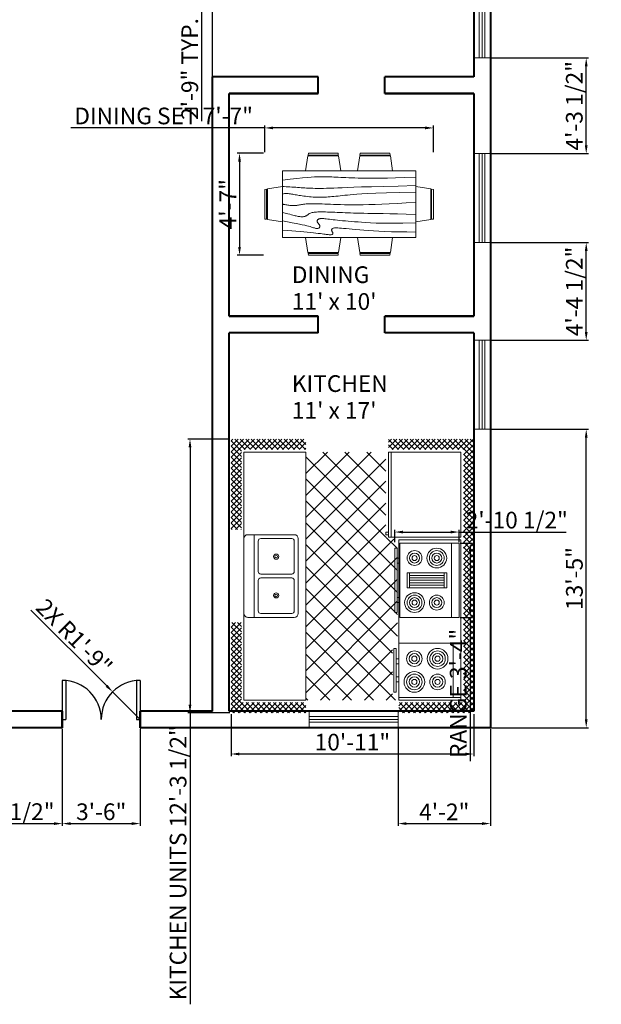
# Model space of a CAD drawing. Units: inches. Extents: x 2383 to 6214, y 970 to 3250.
# Tile 2 of 4: x 2680 to 2994, y 970 to 1500. Entities that reach past the tile are written whole.
import ezdxf

# ---------------------------------------------------------------- set-up
doc = ezdxf.new("R2010")
doc.units = ezdxf.units.IN
for name, color, linetype, lineweight in [('A-ANNO-DIMS', 2, 'Continuous', 18), ('A-AREA-IDEN', 7, 'Continuous', 18), ('A-DOOR', 4, 'Continuous', 25), ('A-EQPM', 8, 'Continuous', 18), ('A-FLOR-FIXT', 8, 'Continuous', 18), ('A-FURN', 8, 'Continuous', 18), ('A-GLAZ', 4, 'Continuous', 18), ('A-WALL', 7, 'Continuous', 40)]:
    doc.layers.add(name, color=color, linetype=linetype, lineweight=lineweight)
doc.styles.get("Standard").update_dxf_attribs({"font": 'arial.ttf'})
doc.dimstyles.new('ISO-25', dxfattribs={"dimtxt": 9, "dimasz": 4.5, "dimexe": 1.25, "dimexo": 0.625, "dimtad": 1, "dimdec": 0, "dimlunit": 3, "dimtxsty": 'Standard', "dimcen": 2.5, "dimadec": 0, "dimazin": 0, "dimtfac": 1, "dimtdec": 0, "dimtmove": 0, "dimatfit": 3, "dimfxl": 1, "dimarcsym": 0})

# ---------------------------------------------------------------- blocks, each defined once
blk = doc.blocks.new('Dining Set - 36 x 72 in.')
for p, q in [((-22, 27.5), (-22.1562, 26.50042)), ((-22, 27.5), (-6, 27.5)), ((-5.8437, 26.49966), (-6, 27.5)), ((6, 27.5), (5.8438, 26.50042)), ((6, 27.5), (22, 27.5)), ((22.1563, 26.49966), (22, 27.5)), ((-22.2343, 26.00059), (-23.4847, 17.99762)), ((-22.2304, 26), (-5.7608, 26)), ((-5.8416, 26.5), (-22.1534, 26.5)), ((-4.5152, 17.99762), (-5.7655, 25.99926)), ((5.7657, 26.00059), (4.5153, 17.99762)), ((5.7696, 26), (22.2392, 26)), ((22.1584, 26.5), (5.8466, 26.5)), ((23.4848, 17.99762), (22.2345, 25.99926)), ((36, 18), (-36, 18)), ((-36, 18), (-36, -18)), ((36, -18), (36, 18)), ((-45.5, 8), (-44.5004, 8.15617)), ((-45.5, 8), (-45.5, -8)), ((-44.5, -8.15843), (-44.5, 8.15338)), ((-44.0006, 8.23428), (-35.9976, 9.48474)), ((-44, 8.23041), (-44, -8.23915)), ((44.0006, 8.23428), (35.9976, 9.48474)), ((44, 8.23041), (44, -8.23915)), ((44.5, -8.15843), (44.5, 8.15338)), ((45.5, 8), (44.5005, 8.15617)), ((45.5, 8), (45.5, -8)), ((-44.4997, -8.15631), (-45.5, -8)), ((-35.9976, -9.48476), (-43.9993, -8.2345)), ((35.9976, -9.48476), (43.9993, -8.2345)), ((44.4997, -8.15631), (45.5, -8)), ((-36, -18), (36, -18)), ((-22.2343, -26.0006), (-23.4847, -17.99762)), ((-4.5152, -17.99762), (-5.7655, -25.99928)), ((5.7657, -26.0006), (4.5153, -17.99762)), ((23.4848, -17.99762), (22.2345, -25.99928)), ((-22.2304, -26), (-5.7608, -26)), ((-22, -27.5), (-22.1562, -26.50044)), ((-5.8416, -26.5), (-22.1534, -26.5)), ((-5.8437, -26.49967), (-6, -27.5)), ((5.7696, -26), (22.2392, -26)), ((6, -27.5), (5.8438, -26.50044)), ((22.1584, -26.5), (5.8466, -26.5)), ((22.1563, -26.49967), (22, -27.5)), ((-22, -27.5), (-6, -27.5)), ((6, -27.5), (22, -27.5))]:
    blk.add_line(p, q)
for points in [[(-36, 15), (-31.1772, 14.97754), (-26.8079, 14.91406), (-22.8538, 14.81543), (-19.276, 14.6875), (-16.0362, 14.53613), (-13.0957, 14.36718), (-10.4159, 14.18652), (-7.9583, 14), (-5.6904, 13.81315), (-3.6035, 13.63021), (-1.6954, 13.45508), (0.0365, 13.29166), (1.5945, 13.14388), (2.9811, 13.01562), (4.1988, 12.9108), (5.25, 12.83333), (6.1393, 12.78613), (6.8802, 12.76823), (7.4883, 12.77767), (7.9792, 12.8125), (8.3685, 12.87077), (8.6719, 12.95052), (8.9049, 13.0498), (9.0833, 13.16666), (9.2205, 13.29899), (9.3216, 13.44401), (9.3895, 13.59879), (9.4271, 13.76041), (9.4373, 13.92594), (9.4232, 14.09245), (9.3875, 14.257), (9.3333, 14.41666), (9.2638, 14.56917), (9.1836, 14.71484), (9.0975, 14.85465), (9.0104, 14.98958), (8.9272, 15.1206), (8.8529, 15.2487), (8.7922, 15.37483), (8.75, 15.5), (8.7305, 15.62467), (8.7344, 15.74739), (8.7617, 15.86621), (8.8125, 15.97916), (8.8867, 16.08431), (8.9844, 16.17968), (9.1055, 16.26334), (9.25, 16.33333), (9.4189, 16.38802), (9.6172, 16.42708), (9.8506, 16.45052), (10.125, 16.45833), (10.4463, 16.45052), (10.8203, 16.42708), (11.2529, 16.38802), (11.75, 16.33333), (12.3184, 16.26318), (12.9694, 16.17838), (13.7151, 16.07991), (14.5677, 15.96875), (15.5395, 15.84586), (16.6426, 15.71224), (17.8893, 15.56884), (19.2917, 15.41666), (20.859, 15.25667), (22.5879, 15.08984), (24.4721, 14.91715), (26.5052, 14.73958), (28.6809, 14.5581), (30.9929, 14.3737), (33.4347, 14.18733), (36, 14)], [(-36, 10), (-28.9766, 10.14274), (-23.1725, 10.20442), (-18.4241, 10.19775), (-14.5677, 10.13541), (-11.4399, 10.03011), (-8.877, 9.89453), (-6.7154, 9.74137), (-4.7917, 9.58333), (-2.9698, 9.43082), (-1.2246, 9.28515), (0.4415, 9.14534), (2.026, 9.01041), (3.5266, 8.87939), (4.9408, 8.7513), (6.266, 8.62516), (7.5, 8.5), (8.6411, 8.37549), (9.6914, 8.2539), (10.6538, 8.13818), (11.5312, 8.03125), (12.3267, 7.93603), (13.043, 7.85547), (13.6831, 7.79248), (14.25, 7.75), (14.7471, 7.7303), (15.1797, 7.73307), (15.5537, 7.75732), (15.875, 7.80208), (16.1494, 7.86637), (16.3828, 7.94922), (16.5811, 8.04964), (16.75, 8.16666), (16.8944, 8.29915), (17.0143, 8.44531), (17.1089, 8.60319), (17.1771, 8.77083), (17.218, 8.94629), (17.2305, 9.1276), (17.2137, 9.31282), (17.1667, 9.5), (17.0895, 9.6875), (16.987, 9.875), (16.8649, 10.0625), (16.7292, 10.25), (16.5856, 10.4375), (16.4401, 10.625), (16.2985, 10.8125), (16.1667, 11), (16.05, 11.18733), (15.9518, 11.3737), (15.8752, 11.5581), (15.8229, 11.73958), (15.798, 11.91715), (15.8034, 12.08984), (15.842, 12.25667), (15.9167, 12.41666), (16.0295, 12.56836), (16.1784, 12.70833), (16.3605, 12.83268), (16.5729, 12.9375), (16.8127, 13.01888), (17.0768, 13.07291), (17.3625, 13.0957), (17.6667, 13.08333), (17.9894, 13.03312), (18.3418, 12.94726), (18.7382, 12.82918), (19.1927, 12.68229), (19.7195, 12.51001), (20.3327, 12.31575), (21.0465, 12.10294), (21.875, 11.875), (22.8357, 11.63354), (23.959, 11.37304), (25.2786, 11.08618), (26.8282, 10.76562), (28.6414, 10.40405), (30.752, 9.99414), (33.1936, 9.52856), (36, 9)], [(-36, 5.5), (-30.7157, 5.3348), (-26.069, 5.20963), (-21.9946, 5.11767), (-18.4271, 5.05208), (-15.3009, 5.00602), (-12.5508, 4.97265), (-10.1112, 4.94515), (-7.9167, 4.91666), (-5.909, 4.88167), (-4.0586, 4.83984), (-2.3429, 4.79215), (-0.7396, 4.73958), (0.7739, 4.6831), (2.22, 4.6237), (3.6213, 4.56233), (5, 4.5), (6.373, 4.43782), (7.7344, 4.3776), (9.0723, 4.32129), (10.375, 4.27083), (11.6309, 4.22819), (12.8281, 4.19531), (13.9551, 4.17415), (15, 4.16666), (15.954, 4.17448), (16.819, 4.19791), (17.6001, 4.23698), (18.3021, 4.29166), (18.9299, 4.36198), (19.4883, 4.44791), (19.9823, 4.54948), (20.4167, 4.66666), (20.7969, 4.79899), (21.1302, 4.94401), (21.4245, 5.09879), (21.6875, 5.26041), (21.9271, 5.42594), (22.1511, 5.59245), (22.3672, 5.757), (22.5834, 5.91666), (22.8065, 6.06868), (23.0404, 6.21093), (23.2879, 6.34147), (23.5521, 6.45833), (23.8358, 6.55957), (24.142, 6.64323), (24.4735, 6.70735), (24.8334, 6.75), (25.2235, 6.76969), (25.642, 6.76692), (26.0858, 6.74267), (26.5521, 6.69791), (27.0379, 6.63362), (27.5404, 6.55078), (28.0565, 6.45036), (28.5834, 6.33333), (29.1242, 6.19987), (29.7071, 6.04687), (30.3661, 5.87044), (31.1354, 5.66666), (32.0493, 5.43164), (33.142, 5.16146), (34.4475, 4.85221), (36, 4.5)], [(-36, -1), (-30.7915, -0.6591), (-26.0195, -0.38216), (-21.6519, -0.16284), (-17.6563, 0.00521), (-14.0005, 0.12833), (-10.6523, 0.21289), (-7.5796, 0.26522), (-4.75, 0.29166), (-2.134, 0.29793), (0.2878, 0.28711), (2.5317, 0.26163), (4.6146, 0.22396), (6.5529, 0.17651), (8.3633, 0.12174), (10.0623, 0.06209), (11.6667, 0), (13.1899, -0.06201), (14.6341, -0.1211), (15.9982, -0.17432), (17.2813, -0.21875), (18.4823, -0.25147), (19.6003, -0.26953), (20.6343, -0.27002), (21.5834, -0.25), (22.4481, -0.20768), (23.2357, -0.14584), (23.9549, -0.06836), (24.6146, 0.02083), (25.2235, 0.11784), (25.7904, 0.21875), (26.3241, 0.31966), (26.8334, 0.41666), (27.3265, 0.50618), (27.8099, 0.58593), (28.2894, 0.65397), (28.7709, 0.70833), (29.2601, 0.74707), (29.763, 0.76823), (30.2855, 0.76985), (30.8334, 0.75), (31.4088, 0.70784), (31.9994, 0.64713), (32.589, 0.57275), (33.1615, 0.48958), (33.7008, 0.4025), (34.1908, 0.3164), (34.6153, 0.23616), (34.9584, 0.16666), (35.2099, 0.11165), (35.3848, 0.07031), (35.504, 0.04069), (35.5886, 0.02083), (35.6594, 0.00879), (35.7377, 0.0026), (35.8442, 0.00032), (36, 0)], [(-36, -6.5), (-27.1843, -6.31267), (-20.084, -6.1263), (-14.469, -5.9419), (-10.1094, -5.76042), (-6.7752, -5.58285), (-4.2363, -5.41016), (-2.2629, -5.24333), (-0.625, -5.08334), (0.8708, -4.93099), (2.2715, -4.78646), (3.5872, -4.64974), (4.8281, -4.52084), (6.0046, -4.39974), (7.127, -4.28646), (8.2053, -4.18099), (9.25, -4.08334), (10.2705, -3.99382), (11.2734, -3.91407), (12.2647, -3.84603), (13.25, -3.79167), (14.2354, -3.75293), (15.2266, -3.73177), (16.2295, -3.73015), (17.25, -3.75), (18.2912, -3.79248), (19.3451, -3.85547), (20.4009, -3.93604), (21.4479, -4.03125), (22.4754, -4.13819), (23.4727, -4.25391), (24.4289, -4.37549), (25.3334, -4.5), (26.1785, -4.62492), (26.9694, -4.74935), (27.7145, -4.87281), (28.4219, -4.99479), (29.1, -5.11483), (29.7572, -5.23242), (30.4016, -5.34709), (31.0417, -5.45834), (31.6837, -5.56437), (32.3262, -5.65821), (32.9658, -5.73153), (33.599, -5.77604), (34.2224, -5.78345), (34.8327, -5.74545), (35.4264, -5.65373), (36, -5.5)], [(-36, -10), (-26.4022, -9.81299), (-18.4675, -9.62891), (-11.9839, -9.45069), (-6.7396, -9.28125), (-2.5226, -9.12354), (0.8789, -8.98047), (3.6769, -8.85498), (6.0833, -8.75), (8.2767, -8.66765), (10.3021, -8.60677), (12.1712, -8.56543), (13.8958, -8.54167), (15.4876, -8.53353), (16.9583, -8.53907), (18.3197, -8.55632), (19.5834, -8.58334), (20.7616, -8.61841), (21.8685, -8.66081), (22.9188, -8.71004), (23.9271, -8.76563), (24.9081, -8.82707), (25.8763, -8.89388), (26.8465, -8.96558), (27.8334, -9.04167), (28.8474, -9.12118), (29.8828, -9.20117), (30.93, -9.27824), (31.9792, -9.34896), (33.0205, -9.40991), (34.0443, -9.45768), (35.0407, -9.48885), (36, -9.5)], [(-36, -14.5), (-30.0881, -14.33513), (-25.0332, -14.21224), (-20.7312, -14.12647), (-17.0781, -14.07292), (-13.97, -14.04671), (-11.3027, -14.04297), (-8.9724, -14.05681), (-6.875, -14.08334), (-4.9224, -14.11833), (-3.0905, -14.16016), (-1.3709, -14.20785), (0.2448, -14.26042), (1.7647, -14.3169), (3.1973, -14.3763), (4.5507, -14.43767), (5.8333, -14.5), (7.0554, -14.5621), (8.235, -14.62175), (9.3922, -14.67652), (10.5469, -14.72396), (11.7192, -14.76164), (12.929, -14.78711), (14.1965, -14.79794), (15.5417, -14.79167), (16.9933, -14.76424), (18.6152, -14.70508), (20.4804, -14.60197), (22.6615, -14.44271), (25.2312, -14.21509), (28.2624, -13.9069), (31.8277, -13.50594), (36, -13)]]:
    blk.add_lwpolyline(points)
blk = doc.blocks.new('Kitchen Layout - 7 x 8 ft')
for p, q in [((-5, 81.32), (2.68, 89)), ((-5, 83.44), (0.56, 89)), ((-5, 85.56), (-1.56, 89)), ((-5, 87.68), (-3.68, 89)), ((-1, 84.97), (-5, 88.97)), ((1.09, 85), (-2.91, 89)), ((3.21, 85), (-0.79, 89)), ((0.81, 85), (4.81, 89)), ((5.34, 85), (1.34, 89)), ((2.93, 85), (6.93, 89)), ((7.46, 85), (3.46, 89)), ((5.05, 85), (9.05, 89)), ((9.58, 85), (5.58, 89)), ((7.17, 85), (11.17, 89)), ((11.7, 85), (7.7, 89)), ((9.29, 85), (13.29, 89)), ((13.82, 85), (9.82, 89)), ((11.41, 85), (15.41, 89)), ((15.94, 85), (11.94, 89)), ((13.53, 85), (17.53, 89)), ((18.06, 85), (14.06, 89)), ((15.65, 85), (19.65, 89)), ((20.18, 85), (16.18, 89)), ((17.78, 85), (21.78, 89)), ((22.31, 85), (18.31, 89)), ((19.9, 85), (23.9, 89)), ((24.43, 85), (20.43, 89)), ((22.02, 85), (26.02, 89)), ((26.55, 85), (22.55, 89)), ((24.14, 85), (28.14, 89)), ((28.67, 85), (24.67, 89)), ((26.26, 85), (30.26, 89)), ((30.79, 85), (26.79, 89)), ((28.38, 85), (32.38, 89)), ((32.91, 85), (28.91, 89)), ((30.5, 85), (34.5, 89)), ((35.03, 85), (31.03, 89)), ((32.63, 85), (36.63, 89)), ((37.16, 85), (33.16, 89)), ((34.75, 85), (38.75, 89)), ((39.28, 85), (35.28, 89)), ((36.87, 85), (40.87, 89)), ((41.4, 85), (37.4, 89)), ((38.99, 85), (42.99, 89)), ((43.52, 85), (39.52, 89)), ((41.11, 85), (45.11, 89)), ((45.64, 85), (41.64, 89)), ((43.23, 85), (47.23, 89)), ((47.76, 85), (43.76, 89)), ((45.35, 85), (49.35, 89)), ((49.88, 85), (45.88, 89)), ((47.47, 85), (51.47, 89)), ((52, 85), (48, 89)), ((49.6, 85), (53.6, 89)), ((54.13, 85), (50.13, 89)), ((51.72, 85), (55.72, 89)), ((56.25, 85), (52.25, 89)), ((53.84, 85), (57.84, 89)), ((58.37, 85), (54.37, 89)), ((55.96, 85), (59.96, 89)), ((60.49, 85), (56.49, 89)), ((58.08, 85), (62.08, 89)), ((62.61, 85), (58.61, 89)), ((60.2, 85), (64.2, 89)), ((64.73, 85), (60.73, 89)), ((62.32, 85), (66.32, 89)), ((66.85, 85), (62.85, 89)), ((64.45, 85), (68.45, 89)), ((68.97, 85), (64.97, 89)), ((66.57, 85), (70.57, 89)), ((71.1, 85), (67.1, 89)), ((68.69, 85), (72.69, 89)), ((73.22, 85), (69.22, 89)), ((70.81, 85), (74.81, 89)), ((75.34, 85), (71.34, 89)), ((72.93, 85), (76.93, 89)), ((77.46, 85), (73.46, 89)), ((75.05, 85), (79.05, 89)), ((79.58, 85), (75.58, 89)), ((77.17, 85), (81.17, 89)), ((81.7, 85), (77.7, 89)), ((79.29, 85), (83.29, 89)), ((83.82, 85), (79.82, 89)), ((81.42, 85), (85.42, 89)), ((85.95, 85), (81.95, 89)), ((83.54, 85), (87.54, 89)), ((88.07, 85), (84.07, 89)), ((85.66, 85), (89.66, 89)), ((90.19, 85), (86.19, 89)), ((87.78, 85), (91.78, 89)), ((92.31, 85), (88.31, 89)), ((89.9, 85), (93.9, 89)), ((94.43, 85), (90.43, 89)), ((92.02, 85), (96.02, 89)), ((96.55, 85), (92.55, 89)), ((94.14, 85), (98.14, 89)), ((101, 82.67), (94.67, 89)), ((96.27, 85), (100.27, 89)), ((101, 84.79), (96.79, 89)), ((101, 86.92), (98.92, 89)), ((-1, 82.85), (-5, 86.85)), ((-1, 80.73), (-5, 84.73)), ((34, 84), (96, 84)), ((34, 60), (34, 84)), ((96, 84), (96, 60)), ((97, 83.61), (101, 87.61)), ((97, 81.49), (101, 85.49)), ((101, 80.55), (97, 84.55)), ((-5, 79.19), (-1, 83.19)), ((-1, 78.61), (-5, 82.61)), ((-5, 77.07), (-1, 81.07)), ((-1, 76.49), (-5, 80.49)), ((74, 81), (95, 81)), ((97, 79.37), (101, 83.37)), ((101, 78.43), (97, 82.43)), ((97, 77.25), (101, 81.25)), ((101, 76.31), (97, 80.31)), ((-5, 74.95), (-1, 78.95)), ((-1, 74.36), (-5, 78.36)), ((-5, 72.83), (-1, 76.83)), ((-1, 72.24), (-5, 76.24)), ((97, 75.13), (101, 79.13)), ((101, 74.19), (97, 78.19)), ((97, 73.01), (101, 77.01)), ((-5, 70.71), (-1, 74.71)), ((-1, 70.12), (-5, 74.12)), ((-5, 68.59), (-1, 72.59)), ((101, 72.07), (97, 76.07)), ((97, 70.89), (101, 74.89)), ((101, 69.95), (97, 73.95)), ((97, 68.76), (101, 72.76)), ((-1, 68), (-5, 72)), ((-5, 66.47), (-1, 70.47)), ((-1, 65.88), (-5, 69.88)), ((101, 67.82), (97, 71.82)), ((97, 66.64), (101, 70.64)), ((101, 65.7), (97, 69.7)), ((-5, 64.35), (-1, 68.35)), ((-1, 63.76), (-5, 67.76)), ((-5, 62.22), (-1, 66.22)), ((-1, 61.64), (-5, 65.64)), ((97, 64.52), (101, 68.52)), ((101, 63.58), (97, 67.58)), ((97, 62.4), (101, 66.4)), ((101, 61.46), (97, 65.46)), ((-5, 60.1), (-1, 64.1)), ((-1, 59.52), (-5, 63.52)), ((-5, 57.98), (-1, 61.98)), ((-1, 57.39), (-5, 61.39)), ((97, 60.28), (101, 64.28)), ((100.34, 60), (97, 63.34)), ((98.22, 60), (97, 61.22)), ((98.84, 60), (101, 62.16)), ((-1.73, 56), (-5, 59.27)), ((-4.86, 56), (-1, 59.86)), ((-2.74, 56), (-1, 57.74)), ((10.4, 24), (45.9, 59.5)), ((18.88, 24), (54.38, 59.5)), ((27.37, 24), (62.87, 59.5)), ((33.03, 55.11), (37.41, 59.5)), ((67.71, 24), (33.68, 58.04)), ((96, 60), (34, 60)), ((35.85, 24), (71.35, 59.5)), ((76.2, 24), (40.7, 59.5)), ((44.34, 24), (77.84, 57.5)), ((84.68, 24), (49.18, 59.5)), ((52.82, 24), (86.32, 57.5)), ((93.17, 24), (57.67, 59.5)), ((61.31, 24), (96, 58.69)), ((96, 29.65), (66.15, 59.5)), ((96, 38.14), (76.64, 57.5)), ((80, 60), (80, 59)), ((82, 59), (82, 60)), ((96, 46.63), (85.13, 57.5)), ((87, 59), (87, 60)), ((89, 60), (89, 59)), ((96, 55.11), (93.57, 57.54)), ((100.96, 60), (101, 60.04)), ((-3.85, 56), (-5, 57.15)), ((0, 57), (33, 57)), ((0, 30.57), (24.43, 55)), ((0, 39.06), (15.94, 55)), ((0, 47.54), (7.46, 55)), ((1.91, 24), (32.91, 55)), ((33.77, 24), (2.77, 55)), ((42.26, 24), (11.26, 55)), ((50.74, 24), (19.74, 55)), ((59.23, 24), (28.23, 55)), ((31, 55), (31, 56)), ((32, 55), (31, 55)), ((32, 56), (32, 55)), ((69.79, 24), (96, 50.21)), ((25.29, 24), (0, 49.29)), ((16.8, 24), (0, 40.8)), ((78.28, 24), (96, 41.72)), ((8.32, 24), (0, 32.32)), ((86.76, 24), (96, 33.24)), ((-5, 21.92), (-2.92, 24)), ((-5, 19.8), (-1, 23.8)), ((-1, 19.21), (-5, 23.21)), ((-1, 21.33), (-3.67, 24)), ((-1, 23.45), (-1.55, 24)), ((0, 24), (96, 24)), ((0, 0), (0, 24)), ((95.25, 24), (96, 24.75)), ((96, 24), (96, 0)), ((97, 22.1), (98.9, 24)), ((97, 19.97), (101, 23.97)), ((101, 19.03), (97, 23.03)), ((101, 21.16), (98.16, 24)), ((101, 23.28), (100.28, 24)), ((-5, 17.68), (-1, 21.68)), ((-1, 17.09), (-5, 21.09)), ((-5, 15.55), (-1, 19.55)), ((97, 17.85), (101, 21.85)), ((101, 16.91), (97, 20.91)), ((97, 15.73), (101, 19.73)), ((-1, 14.97), (-5, 18.97)), ((-5, 13.43), (-1, 17.43)), ((-1, 12.85), (-5, 16.85)), ((-5, 11.31), (-1, 15.31)), ((47.25, 6.5), (47.25, 18.5)), ((48.75, 18.5), (48.75, 6.5)), ((101, 14.79), (97, 18.79)), ((97, 13.61), (101, 17.61)), ((101, 12.67), (97, 16.67)), ((97, 11.49), (101, 15.49)), ((-1, 10.73), (-5, 14.73)), ((-5, 9.19), (-1, 13.19)), ((-1, 8.6), (-5, 12.6)), ((101, 10.55), (97, 14.55)), ((97, 9.37), (101, 13.37)), ((101, 8.43), (97, 12.43)), ((-5, 7.07), (-1, 11.07)), ((-1, 6.48), (-5, 10.48)), ((-5, 4.95), (-1, 8.95)), ((-1, 4.36), (-5, 8.36)), ((97, 7.25), (101, 11.25)), ((101, 6.31), (97, 10.31)), ((97, 5.12), (101, 9.12)), ((101, 4.18), (97, 8.18)), ((-5, 2.83), (-1, 6.83)), ((-1, 2.24), (-5, 6.24)), ((-5, 0.71), (-1, 4.71)), ((-1, 0.12), (-5, 4.12)), ((64, 4), (32, 4)), ((97, 3), (101, 7)), ((101, 2.06), (97, 6.06)), ((97, 0.88), (101, 4.88)), ((101, -0.06), (97, 3.94)), ((-5, -1.42), (-1, 2.58)), ((2, -5), (-5, 2)), ((-5, -3.54), (-1, 0.46)), ((96, 0), (0, 0)), ((93.24, -5), (101, 2.76)), ((95.36, -5), (101, 0.64)), ((101, -2.18), (97, 1.82)), ((-0.12, -5), (-5, -0.12)), ((-2.25, -5), (-5, -2.25)), ((-4.34, -5), (-0.34, -1)), ((-2.22, -5), (1.78, -1)), ((-0.1, -5), (3.9, -1)), ((4.12, -5), (0.12, -1)), ((2.02, -5), (6.02, -1)), ((6.24, -5), (2.24, -1)), ((4.14, -5), (8.14, -1)), ((8.36, -5), (4.36, -1)), ((6.27, -5), (10.27, -1)), ((10.48, -5), (6.48, -1)), ((8.39, -5), (12.39, -1)), ((12.6, -5), (8.6, -1)), ((10.51, -5), (14.51, -1)), ((14.73, -5), (10.73, -1)), ((12.63, -5), (16.63, -1)), ((16.85, -5), (12.85, -1)), ((14.75, -5), (18.75, -1)), ((18.97, -5), (14.97, -1)), ((16.87, -5), (20.87, -1)), ((21.09, -5), (17.09, -1)), ((18.99, -5), (22.99, -1)), ((23.21, -5), (19.21, -1)), ((21.11, -5), (25.11, -1)), ((25.33, -5), (21.33, -1)), ((23.24, -5), (27.24, -1)), ((27.45, -5), (23.45, -1)), ((25.36, -5), (29.36, -1)), ((29.57, -5), (25.57, -1)), ((27.48, -5), (30, -2.48)), ((30, -3.3), (27.7, -1)), ((30, -1.18), (29.82, -1)), ((66, -2.54), (67.54, -1)), ((66, -4.66), (69.66, -1)), ((69.88, -5), (66, -1.12)), ((67.76, -5), (66, -3.24)), ((67.78, -5), (71.78, -1)), ((72, -5), (68, -1)), ((69.9, -5), (73.9, -1)), ((74.12, -5), (70.12, -1)), ((72.03, -5), (76.03, -1)), ((76.24, -5), (72.24, -1)), ((74.15, -5), (78.15, -1)), ((78.36, -5), (74.36, -1)), ((76.27, -5), (80.27, -1)), ((80.49, -5), (76.49, -1)), ((78.39, -5), (82.39, -1)), ((82.61, -5), (78.61, -1)), ((80.51, -5), (84.51, -1)), ((84.73, -5), (80.73, -1)), ((82.63, -5), (86.63, -1)), ((86.85, -5), (82.85, -1)), ((84.75, -5), (88.75, -1)), ((88.97, -5), (84.97, -1)), ((86.88, -5), (90.88, -1)), ((91.09, -5), (87.09, -1)), ((89, -5), (93, -1)), ((93.21, -5), (89.21, -1)), ((91.12, -5), (95.12, -1)), ((95.34, -5), (91.34, -1)), ((97.46, -5), (93.46, -1)), ((99.58, -5), (95.58, -1)), ((101, -4.3), (97, -0.3)), ((97.48, -5), (101, -1.48)), ((99.6, -5), (101, -3.6)), ((-4.37, -5), (-5, -4.37)), ((29.6, -5), (30, -4.6))]:
    blk.add_line(p, q)
for points in [[(0, 56), (0, 84), (33, 84), (33, 56)], [(74, 60), (74, 84), (95, 84), (95, 60)], [(76, 58), (76, 59), (93, 59), (93, 58)]]:
    blk.add_lwpolyline(points, close=True)
for points in [[(32, 1.5), (32, 19.5)], [(33.5, 21), (62.5, 21)], [(34.5, 19.5), (46.25, 19.5)], [(49.75, 19.5), (61.5, 19.5)], [(64, 19.5), (64, 1.5)], [(33.5, 6.5), (33.5, 18.5)], [(62.5, 18.5), (62.5, 6.5)], [(46.25, 5.5), (34.5, 5.5)], [(61.5, 5.5), (49.75, 5.5)], [(62.5, 0), (33.5, 0)]]:
    blk.add_lwpolyline(points)
for centre, radius in [((80, 75), 4), ((80, 75), 3), ((80, 75), 2), ((89, 75), 3), ((89, 75), 2), ((80, 75), 1), ((89, 75), 1), ((80, 66), 3), ((89, 66), 4), ((89, 66), 3), ((80, 66), 2), ((80, 66), 1), ((89, 66), 2), ((89, 66), 1), ((40.5, 12.5), 1), ((40.5, 12.5), 0.5), ((55.5, 12.5), 1), ((55.5, 12.5), 0.5)]:
    blk.add_circle(centre, radius)
for centre, radius, start, end in [((33.5, 19.5), 1.5, 90, 180), ((34.5, 18.5), 1, 90, 180), ((46.25, 18.5), 1, 0, 90), ((49.75, 18.5), 1, 90, 180), ((61.5, 18.5), 1, 0, 90), ((62.5, 19.5), 1.5, 0, 90), ((34.5, 6.5), 1, 180, 270), ((46.25, 6.5), 1, 270, 0), ((49.75, 6.5), 1, 180, 270), ((61.5, 6.5), 1, 270, 0), ((33.5, 1.5), 1.5, 180, 270), ((62.5, 1.5), 1.5, 270, 0)]:
    blk.add_arc(centre, radius, start, end)
blk = doc.blocks.new('Range-Oven - 30 in top')
for p, q in [((0, -3), (30, -3)), ((12, -6), (18, -6)), ((13, -20), (13, -6)), ((14, -6), (14, -20)), ((15, -20), (15, -6)), ((16, -6), (16, -20)), ((17, -20), (17, -6)), ((18, -20), (12, -20)), ((6, -24), (6, -25)), ((8, -25), (8, -24)), ((22, -25), (22, -24)), ((24, -24), (24, -25))]:
    blk.add_line(p, q)
for points in [[(0, -24), (0, 0), (30, 0), (30, -24)], [(12, -21), (12, -5), (18, -5), (18, -21)], [(2, -26), (2, -25), (28, -25), (28, -26)]]:
    blk.add_lwpolyline(points, close=True)
for centre, radius in [((6, -9), 4), ((6, -9), 3), ((6, -9), 2), ((24, -9), 3), ((24, -9), 2), ((6, -9), 1), ((24, -9), 1), ((6, -18), 3), ((24, -18), 4), ((24, -18), 3), ((6, -18), 2), ((6, -18), 1), ((24, -18), 2), ((24, -18), 1)]:
    blk.add_circle(centre, radius)
blk = doc.blocks.new('WINDOW-48X9IN')
for p, q in [((3, 0), (3, 48)), ((4.5, 0), (4.5, 48)), ((6, 0), (6, 48))]:
    blk.add_line(p, q)
blk.add_lwpolyline([(0, 0), (0, 48), (9, 48), (9, 0)], close=True)
blk = doc.blocks.new('*D38')
at = {"layer": 'A-ANNO-DIMS', "color": 0, "lineweight": -2, "transparency": 16777216}
for p, q in [((2783.33, 1539.35), (2776.74, 1539.35)), ((2777.99, 1534.85), (2777.99, 1511.02)), ((2783.33, 1506.52), (2776.74, 1506.52)), ((2777.99, 1506.52), (2777.99, 1445.76))]:
    blk.add_line(p, q, dxfattribs=at)
at = {"layer": 'A-ANNO-DIMS', "color": 0, "transparency": 16777216}
for points in [[(2777.24, 1534.85), (2778.74, 1534.85), (2777.99, 1539.35)], [(2777.24, 1511.02), (2778.74, 1511.02), (2777.99, 1506.52)]]:
    blk.add_solid(points, dxfattribs=at)
at = {"layer": 'Defpoints', "color": 0, "transparency": 16777216}
for p in [(2783.96, 1539.35), (2777.99, 1506.52), (2783.96, 1506.52)]:
    blk.add_point(p, dxfattribs=at)
at = {"layer": 'A-ANNO-DIMS', "color": 0, "transparency": 16777216, "insert": (2772.77, 1473.89), "char_height": 9, "attachment_point": 5, "rotation": 90}
blk.add_mtext('2\'-9" TYP.', dxfattribs=at)
blk = doc.blocks.new('*D43')
at = {"layer": 'A-ANNO-DIMS', "color": 0, "lineweight": -2, "transparency": 16777216}
for p, q in [((2812.1, 1442.14), (2707.43, 1442.14)), ((2812.1, 1429.12), (2812.1, 1443.39)), ((2898.6, 1442.14), (2816.6, 1442.14)), ((2903.1, 1429.12), (2903.1, 1443.39))]:
    blk.add_line(p, q, dxfattribs=at)
at = {"layer": 'A-ANNO-DIMS', "color": 0, "transparency": 16777216}
for points in [[(2816.6, 1442.89), (2816.6, 1441.39), (2812.1, 1442.14)], [(2898.6, 1442.89), (2898.6, 1441.39), (2903.1, 1442.14)]]:
    blk.add_solid(points, dxfattribs=at)
at = {"layer": 'Defpoints', "color": 0, "transparency": 16777216}
for p in [(2812.1, 1442.14), (2812.1, 1428.49), (2903.1, 1428.49)]:
    blk.add_point(p, dxfattribs=at)
at = {"layer": 'A-ANNO-DIMS', "color": 0, "transparency": 16777216, "insert": (2757.51, 1447.42), "char_height": 9, "attachment_point": 5}
blk.add_mtext('DINING SET 7\'-7"', dxfattribs=at)
blk = doc.blocks.new('*D44')
at = {"layer": 'A-ANNO-DIMS', "color": 0, "lineweight": -2, "transparency": 16777216}
for p, q in [((2811.47, 1428.49), (2797.2, 1428.49)), ((2798.45, 1423.99), (2798.45, 1377.99)), ((2811.47, 1373.49), (2797.2, 1373.49))]:
    blk.add_line(p, q, dxfattribs=at)
at = {"layer": 'A-ANNO-DIMS', "color": 0, "transparency": 16777216}
for points in [[(2797.7, 1423.99), (2799.2, 1423.99), (2798.45, 1428.49)], [(2797.7, 1377.99), (2799.2, 1377.99), (2798.45, 1373.49)]]:
    blk.add_solid(points, dxfattribs=at)
at = {"layer": 'Defpoints', "color": 0, "transparency": 16777216}
for p in [(2812.1, 1428.49), (2798.45, 1373.49), (2812.1, 1373.49)]:
    blk.add_point(p, dxfattribs=at)
at = {"layer": 'A-ANNO-DIMS', "color": 0, "transparency": 16777216, "insert": (2793.32, 1400.99), "char_height": 9, "attachment_point": 5, "rotation": 90}
blk.add_mtext('4\'-7"', dxfattribs=at)
blk = doc.blocks.new('*D47')
at = {"layer": 'A-ANNO-DIMS', "color": 0, "lineweight": -2, "transparency": 16777216}
for p, q in [((2793.26, 1274.31), (2770.49, 1274.31)), ((2771.74, 1269.81), (2771.74, 1131.16)), ((2793.26, 1126.66), (2770.49, 1126.66)), ((2771.74, 1126.66), (2771.74, 969.53))]:
    blk.add_line(p, q, dxfattribs=at)
at = {"layer": 'A-ANNO-DIMS', "color": 0, "transparency": 16777216}
for points in [[(2770.99, 1269.81), (2772.49, 1269.81), (2771.74, 1274.31)], [(2770.99, 1131.16), (2772.49, 1131.16), (2771.74, 1126.66)]]:
    blk.add_solid(points, dxfattribs=at)
at = {"layer": 'Defpoints', "color": 0, "transparency": 16777216}
for p in [(2793.89, 1274.31), (2771.74, 1126.66), (2793.89, 1126.66)]:
    blk.add_point(p, dxfattribs=at)
at = {"layer": 'A-ANNO-DIMS', "color": 0, "transparency": 16777216, "insert": (2766.46, 1045.84), "char_height": 9, "attachment_point": 5, "rotation": 90}
blk.add_mtext('KITCHEN UNITS 12\'-3 1/2"', dxfattribs=at)
blk = doc.blocks.new('*D48')
at = {"layer": 'A-ANNO-DIMS', "color": 0, "lineweight": -2, "transparency": 16777216}
for p, q in [((2793.89, 1126.03), (2793.89, 1103.26)), ((2924.83, 1126.03), (2924.83, 1103.26)), ((2798.39, 1104.51), (2920.33, 1104.51))]:
    blk.add_line(p, q, dxfattribs=at)
at = {"layer": 'A-ANNO-DIMS', "color": 0, "transparency": 16777216}
for points in [[(2798.39, 1105.26), (2798.39, 1103.76), (2793.89, 1104.51)], [(2920.33, 1105.26), (2920.33, 1103.76), (2924.83, 1104.51)]]:
    blk.add_solid(points, dxfattribs=at)
at = {"layer": 'Defpoints', "color": 0, "transparency": 16777216}
for p in [(2793.89, 1126.66), (2924.83, 1126.66), (2924.83, 1104.51)]:
    blk.add_point(p, dxfattribs=at)
at = {"layer": 'A-ANNO-DIMS', "color": 0, "transparency": 16777216, "insert": (2859.36, 1109.73), "char_height": 9, "attachment_point": 5}
blk.add_mtext('10\'-11"', dxfattribs=at)
blk = doc.blocks.new('*D49')
at = {"layer": 'A-ANNO-DIMS', "color": 0, "lineweight": -2, "transparency": 16777216}
for p, q in [((2917.53, 1218.18), (2924.16, 1218.18)), ((2922.91, 1213.68), (2922.91, 1182.64)), ((2917.53, 1178.14), (2924.16, 1178.14)), ((2922.91, 1178.14), (2922.91, 1100.73))]:
    blk.add_line(p, q, dxfattribs=at)
at = {"layer": 'A-ANNO-DIMS', "color": 0, "transparency": 16777216}
for points in [[(2922.16, 1213.68), (2923.66, 1213.68), (2922.91, 1218.18)], [(2922.16, 1182.64), (2923.66, 1182.64), (2922.91, 1178.14)]]:
    blk.add_solid(points, dxfattribs=at)
at = {"layer": 'Defpoints', "color": 0, "transparency": 16777216}
for p in [(2916.91, 1218.18), (2916.91, 1178.14), (2922.91, 1178.14)]:
    blk.add_point(p, dxfattribs=at)
at = {"layer": 'A-ANNO-DIMS', "color": 0, "transparency": 16777216, "insert": (2917.63, 1137.19), "char_height": 9, "attachment_point": 5, "rotation": 90}
blk.add_mtext('RANGE 3\'-4"', dxfattribs=at)
blk = doc.blocks.new('*D50')
at = {"layer": 'A-ANNO-DIMS', "color": 0, "lineweight": -2, "transparency": 16777216}
for p, q in [((2882.21, 1218.81), (2882.21, 1225.44)), ((2886.71, 1224.19), (2912.41, 1224.19)), ((2916.91, 1218.81), (2916.91, 1225.44)), ((2916.91, 1224.19), (2974.7, 1224.19))]:
    blk.add_line(p, q, dxfattribs=at)
at = {"layer": 'A-ANNO-DIMS', "color": 0, "transparency": 16777216}
for points in [[(2886.71, 1224.94), (2886.71, 1223.44), (2882.21, 1224.19)], [(2912.41, 1224.94), (2912.41, 1223.44), (2916.91, 1224.19)]]:
    blk.add_solid(points, dxfattribs=at)
at = {"layer": 'Defpoints', "color": 0, "transparency": 16777216}
for p in [(2916.91, 1224.19), (2882.21, 1218.18), (2916.91, 1218.18)]:
    blk.add_point(p, dxfattribs=at)
at = {"layer": 'A-ANNO-DIMS', "color": 0, "transparency": 16777216, "insert": (2948.05, 1229.46), "char_height": 9, "attachment_point": 5}
blk.add_mtext('2\'-10 1/2"', dxfattribs=at)
blk = doc.blocks.new('*D54')
at = {"layer": 'A-ANNO-DIMS', "color": 0, "lineweight": -2, "transparency": 16777216}
for p, q in [((2646.17, 1118.05), (2646.17, 1065.73)), ((2702.83, 1118.05), (2702.83, 1065.73)), ((2650.67, 1066.98), (2698.33, 1066.98))]:
    blk.add_line(p, q, dxfattribs=at)
at = {"layer": 'A-ANNO-DIMS', "color": 0, "transparency": 16777216}
for points in [[(2650.67, 1067.73), (2650.67, 1066.23), (2646.17, 1066.98)], [(2698.33, 1067.73), (2698.33, 1066.23), (2702.83, 1066.98)]]:
    blk.add_solid(points, dxfattribs=at)
at = {"layer": 'Defpoints', "color": 0, "transparency": 16777216}
for p in [(2646.17, 1118.68), (2702.83, 1118.68), (2702.83, 1066.98)]:
    blk.add_point(p, dxfattribs=at)
at = {"layer": 'A-ANNO-DIMS', "color": 0, "transparency": 16777216, "insert": (2674.5, 1072.26), "char_height": 9, "attachment_point": 5}
blk.add_mtext('4\'-8 1/2"', dxfattribs=at)
blk = doc.blocks.new('*D55')
at = {"layer": 'A-ANNO-DIMS', "color": 0, "lineweight": -2, "transparency": 16777216}
for p, q in [((2702.83, 1118.05), (2702.83, 1065.73)), ((2744.83, 1118.05), (2744.83, 1065.73)), ((2707.33, 1066.98), (2740.33, 1066.98))]:
    blk.add_line(p, q, dxfattribs=at)
at = {"layer": 'A-ANNO-DIMS', "color": 0, "transparency": 16777216}
for points in [[(2707.33, 1067.73), (2707.33, 1066.23), (2702.83, 1066.98)], [(2740.33, 1067.73), (2740.33, 1066.23), (2744.83, 1066.98)]]:
    blk.add_solid(points, dxfattribs=at)
at = {"layer": 'Defpoints', "color": 0, "transparency": 16777216}
for p in [(2702.83, 1118.68), (2744.83, 1118.68), (2744.83, 1066.98)]:
    blk.add_point(p, dxfattribs=at)
at = {"layer": 'A-ANNO-DIMS', "color": 0, "transparency": 16777216, "insert": (2723.83, 1072.2), "char_height": 9, "attachment_point": 5}
blk.add_mtext('3\'-6"', dxfattribs=at)
blk = doc.blocks.new('*D56')
at = {"layer": 'A-ANNO-DIMS', "color": 0, "lineweight": -2, "transparency": 16777216}
for p, q in [((2663.83, 1128.3), (2663.83, 2131.63)), ((2668.33, 2130.38), (2779.33, 2130.38)), ((2783.83, 1128.3), (2783.83, 2131.63))]:
    blk.add_line(p, q, dxfattribs=at)
at = {"layer": 'A-ANNO-DIMS', "color": 0, "transparency": 16777216}
for points in [[(2668.33, 2131.13), (2668.33, 2129.63), (2663.83, 2130.38)], [(2779.33, 2131.13), (2779.33, 2129.63), (2783.83, 2130.38)]]:
    blk.add_solid(points, dxfattribs=at)
at = {"layer": 'Defpoints', "color": 0, "transparency": 16777216}
for p in [(2783.83, 2130.38), (2663.83, 1127.68), (2783.83, 1127.68)]:
    blk.add_point(p, dxfattribs=at)
at = {"layer": 'A-ANNO-DIMS', "color": 0, "transparency": 16777216, "insert": (2723.83, 2135.6), "char_height": 9, "attachment_point": 5}
blk.add_mtext('10\'-0"', dxfattribs=at)
blk = doc.blocks.new('*D57')
at = {"layer": 'A-ANNO-DIMS', "color": 0, "lineweight": -2, "transparency": 16777216}
for p, q in [((2884.04, 1118.05), (2884.04, 1065.73)), ((2933.83, 1118.05), (2933.83, 1065.73)), ((2888.54, 1066.98), (2929.33, 1066.98))]:
    blk.add_line(p, q, dxfattribs=at)
at = {"layer": 'A-ANNO-DIMS', "color": 0, "transparency": 16777216}
for points in [[(2888.54, 1067.73), (2888.54, 1066.23), (2884.04, 1066.98)], [(2929.33, 1067.73), (2929.33, 1066.23), (2933.83, 1066.98)]]:
    blk.add_solid(points, dxfattribs=at)
at = {"layer": 'Defpoints', "color": 0, "transparency": 16777216}
for p in [(2884.04, 1118.68), (2933.83, 1118.68), (2933.83, 1066.98)]:
    blk.add_point(p, dxfattribs=at)
at = {"layer": 'A-ANNO-DIMS', "color": 0, "transparency": 16777216, "insert": (2908.93, 1072.12), "char_height": 9, "attachment_point": 5}
blk.add_mtext('4\'-2"', dxfattribs=at)
blk = doc.blocks.new('*D65')
at = {"layer": 'A-ANNO-DIMS', "color": 0, "lineweight": -2, "transparency": 16777216}
for p, q in [((2934.45, 1279.61), (2986.78, 1279.61)), ((2985.53, 1123.18), (2985.53, 1275.11)), ((2934.45, 1118.68), (2986.78, 1118.68))]:
    blk.add_line(p, q, dxfattribs=at)
at = {"layer": 'A-ANNO-DIMS', "color": 0, "transparency": 16777216}
for points in [[(2984.78, 1275.11), (2986.28, 1275.11), (2985.53, 1279.61)], [(2984.78, 1123.18), (2986.28, 1123.18), (2985.53, 1118.68)]]:
    blk.add_solid(points, dxfattribs=at)
at = {"layer": 'Defpoints', "color": 0, "transparency": 16777216}
for p in [(2933.83, 1279.61), (2985.53, 1279.61), (2933.83, 1118.68)]:
    blk.add_point(p, dxfattribs=at)
at = {"layer": 'A-ANNO-DIMS', "color": 0, "transparency": 16777216, "insert": (2980.3, 1199.14), "char_height": 9, "attachment_point": 5, "rotation": 90}
blk.add_mtext('13\'-5"', dxfattribs=at)
blk = doc.blocks.new('*D66')
at = {"layer": 'A-ANNO-DIMS', "color": 0, "lineweight": -2, "transparency": 16777216}
for p, q in [((2934.45, 1380.27), (2986.78, 1380.27)), ((2985.53, 1332.11), (2985.53, 1375.77)), ((2934.45, 1327.61), (2986.78, 1327.61))]:
    blk.add_line(p, q, dxfattribs=at)
at = {"layer": 'A-ANNO-DIMS', "color": 0, "transparency": 16777216}
for points in [[(2984.78, 1375.77), (2986.28, 1375.77), (2985.53, 1380.27)], [(2984.78, 1332.11), (2986.28, 1332.11), (2985.53, 1327.61)]]:
    blk.add_solid(points, dxfattribs=at)
at = {"layer": 'Defpoints', "color": 0, "transparency": 16777216}
for p in [(2933.83, 1380.27), (2985.53, 1380.27), (2933.83, 1327.61)]:
    blk.add_point(p, dxfattribs=at)
at = {"layer": 'A-ANNO-DIMS', "color": 0, "transparency": 16777216, "insert": (2980.25, 1353.94), "char_height": 9, "attachment_point": 5, "rotation": 90}
blk.add_mtext('4\'-4 1/2"', dxfattribs=at)
blk = doc.blocks.new('*D67')
at = {"layer": 'A-ANNO-DIMS', "color": 0, "lineweight": -2, "transparency": 16777216}
for p, q in [((2934.45, 1479.85), (2986.78, 1479.85)), ((2985.53, 1432.77), (2985.53, 1475.35)), ((2934.45, 1428.27), (2986.78, 1428.27))]:
    blk.add_line(p, q, dxfattribs=at)
at = {"layer": 'A-ANNO-DIMS', "color": 0, "transparency": 16777216}
for points in [[(2984.78, 1475.35), (2986.28, 1475.35), (2985.53, 1479.85)], [(2984.78, 1432.77), (2986.28, 1432.77), (2985.53, 1428.27)]]:
    blk.add_solid(points, dxfattribs=at)
at = {"layer": 'Defpoints', "color": 0, "transparency": 16777216}
for p in [(2933.83, 1479.85), (2985.53, 1479.85), (2933.83, 1428.27)]:
    blk.add_point(p, dxfattribs=at)
at = {"layer": 'A-ANNO-DIMS', "color": 0, "transparency": 16777216, "insert": (2980.25, 1454.06), "char_height": 9, "attachment_point": 5, "rotation": 90}
blk.add_mtext('4\'-3 1/2"', dxfattribs=at)
blk = doc.blocks.new('*D73')
at = {"layer": 'A-ANNO-DIMS', "color": 0, "lineweight": -2, "transparency": 16777216}
for p, q in [((2685.94, 1182.07), (2726.8, 1141.21)), ((2744.83, 1123.18), (2729.98, 1138.03))]:
    blk.add_line(p, q, dxfattribs=at)
at = {"layer": 'A-ANNO-DIMS', "color": 0, "transparency": 16777216}
blk.add_solid([(2727.33, 1141.74), (2726.27, 1140.68), (2729.98, 1138.03)], dxfattribs=at)
at = {"layer": 'Defpoints', "color": 0, "transparency": 16777216}
for p in [(2729.98, 1138.03), (2744.83, 1123.18)]:
    blk.add_point(p, dxfattribs=at)
at = {"layer": 'A-ANNO-DIMS', "color": 0, "transparency": 16777216, "insert": (2708.47, 1166.92), "char_height": 9, "attachment_point": 5, "rotation": 314.9997}
blk.add_mtext('2X R1\'-9"', dxfattribs=at)

msp = doc.modelspace()

# ---------------------------------------------------------------- linework, layer by layer
at = {"layer": 'A-DOOR'}
for p, q in [((2702.83, 1144.18), (2702.83, 1123.18)), ((2704.83, 1144.18), (2704.83, 1123.18)), ((2742.83, 1144.18), (2742.83, 1123.18)), ((2744.83, 1144.18), (2744.83, 1123.18)), ((2702.83, 1123.18), (2704.83, 1123.18)), ((2742.83, 1123.18), (2744.83, 1123.18))]:
    msp.add_line(p, q, dxfattribs=at)
for centre, start, end in [((2702.83, 1123.18), 0, 90), ((2744.83, 1123.18), 90, 180)]:
    msp.add_arc(centre, 21, start, end, dxfattribs=at)
at = {"layer": 'A-WALL'}
for p, q in [((2933.83, 2078.68), (2933.83, 1118.68)), ((2924.83, 1718.68), (2924.83, 1469.68)), ((2783.83, 1127.68), (2783.83, 1469.68)), ((2840.83, 1469.68), (2783.83, 1469.68)), ((2840.83, 1460.68), (2840.83, 1469.68)), ((2924.83, 1469.68), (2876.83, 1469.68)), ((2876.83, 1460.68), (2876.83, 1469.68)), ((2792.83, 1460.68), (2840.83, 1460.68)), ((2840.83, 1460.68), (2792.83, 1460.68)), ((2792.83, 1340.68), (2792.83, 1460.68)), ((2924.83, 1460.68), (2876.83, 1460.68)), ((2876.83, 1460.68), (2924.83, 1460.68)), ((2924.83, 1460.68), (2924.83, 1340.68)), ((2792.83, 1340.68), (2840.83, 1340.68)), ((2840.83, 1340.68), (2792.83, 1340.68)), ((2840.83, 1331.68), (2840.83, 1340.68)), ((2924.83, 1340.68), (2876.83, 1340.68)), ((2876.83, 1331.68), (2876.83, 1340.68)), ((2876.83, 1340.68), (2924.83, 1340.68)), ((2792.83, 1127.68), (2792.83, 1331.68)), ((2840.83, 1331.68), (2792.83, 1331.68)), ((2924.83, 1331.68), (2876.83, 1331.68)), ((2924.83, 1331.68), (2924.83, 1127.68)), ((2702.83, 1127.68), (2663.83, 1127.68)), ((2702.83, 1118.68), (2702.83, 1127.68)), ((2702.83, 1127.68), (2702.83, 1118.68)), ((2783.83, 1127.68), (2744.83, 1127.68)), ((2744.83, 1118.68), (2744.83, 1127.68)), ((2744.83, 1127.68), (2744.83, 1118.68)), ((2924.83, 1127.68), (2792.83, 1127.68)), ((2702.83, 1118.68), (2453.83, 1118.68)), ((2933.83, 1118.68), (2744.83, 1118.68))]:
    msp.add_line(p, q, dxfattribs=at)

# ---------------------------------------------------------------- block references
at = {"layer": 'A-EQPM', "xscale": 1.334555769470256, "yscale": 1.334555769470256, "zscale": 1.334555769470256, "rotation": 270}
msp.add_blockref('Range-Oven - 30 in top', (2916.91, 1218.18), dxfattribs=at)
at = {"layer": 'A-FLOR-FIXT', "xscale": 1.392961780722463, "yscale": 1.392961780722463, "zscale": 1.392961780722463, "rotation": 270}
msp.add_blockref('Kitchen Layout - 7 x 8 ft', (2800.85, 1267.35), dxfattribs=at)
at = {"layer": 'A-FURN', "rotation": 180}
msp.add_blockref('Dining Set - 36 x 72 in.', (2857.6, 1400.99), dxfattribs=at)
at = {"layer": 'A-GLAZ'}
for p in [(2924.83, 1479.85), (2924.83, 1380.27), (2924.83, 1279.61)]:
    msp.add_blockref('WINDOW-48X9IN', p, dxfattribs=at)
at = {"layer": 'A-GLAZ', "rotation": 270.0000000000005}
msp.add_blockref('WINDOW-48X9IN', (2836.04, 1127.68), dxfattribs=at)

# ---------------------------------------------------------------- texts
at = {"layer": 'A-AREA-IDEN'}
for s, p in [('DINING', (2826.68, 1358.49)), ("11' x 10'", (2826.68, 1344.03)), ('KITCHEN', (2826.68, 1299.75)), ("11' x 17'", (2826.68, 1285.29))]:
    msp.add_text(s, height=9, dxfattribs=at).set_placement(p)

# ---------------------------------------------------------------- dimensions: what is measured, and where the dimension line sits
at = {"layer": 'A-ANNO-DIMS'}
for base, p1, p2, picture, middle in [((2783.83, 2130.38), (2663.83, 1127.68), (2783.83, 1127.68), '*D56', (2723.83, 2135.6)), ((2916.91, 1224.19), (2882.21, 1218.18), (2916.91, 1218.18), '*D50', (2948.05, 1229.46)), ((2924.83, 1104.51), (2793.89, 1126.66), (2924.83, 1126.66), '*D48', (2859.36, 1109.73)), ((2702.83, 1066.98), (2646.17, 1118.68), (2702.83, 1118.68), '*D54', (2674.5, 1072.26)), ((2744.83, 1066.98), (2702.83, 1118.68), (2744.83, 1118.68), '*D55', (2723.83, 1072.2)), ((2933.83, 1066.98), (2884.04, 1118.68), (2933.83, 1118.68), '*D57', (2908.93, 1072.12))]:
    dim = msp.add_linear_dim(base=base, p1=p1, p2=p2, dimstyle='ISO-25', override={"dimdec": 1, "dimlfac": 1, "dimrnd": 0, "dimzin": 1, "dimdsep": 46, "dimlunit": 4, "dimfrac": 2}, dxfattribs=at)
    dim.commit()
    dim.dimension.update_dxf_attribs({"geometry": picture, "text_midpoint": middle})
for base, p1, p2, angle, text, picture, middle in [((2777.99, 1506.52), (2783.96, 1539.35), (2783.96, 1506.52), 270, '<> TYP.', '*D38', (2772.77, 1473.89)), ((2812.1, 1442.14), (2903.1, 1428.49), (2812.1, 1428.49), 180, 'DINING SET <>', '*D43', (2757.51, 1447.42)), ((2771.7416, 1126.6561), (2793.8897, 1274.31), (2793.8897, 1126.6561), 270, 'KITCHEN UNITS <>', '*D47', (2766.46, 1045.8414)), ((2922.91, 1178.14), (2916.91, 1218.18), (2916.91, 1178.14), 270, 'RANGE <>', '*D49', (2917.63, 1137.19))]:
    dim = msp.add_linear_dim(base=base, p1=p1, p2=p2, angle=angle, text=text, dimstyle='ISO-25', override={"dimdec": 1, "dimlfac": 1, "dimrnd": 0, "dimzin": 1, "dimdsep": 46, "dimlunit": 4, "dimfrac": 2}, dxfattribs=at)
    dim.commit()
    dim.dimension.update_dxf_attribs({"geometry": picture, "text_midpoint": middle})
for base, p1, p2, angle, picture, middle in [((2985.53, 1479.85), (2933.83, 1428.27), (2933.83, 1479.85), 90, '*D67', (2980.25, 1454.06)), ((2798.45, 1373.49), (2812.1, 1428.49), (2812.1, 1373.49), 270, '*D44', (2793.32, 1400.99)), ((2985.53, 1380.27), (2933.83, 1327.61), (2933.83, 1380.27), 90, '*D66', (2980.25, 1353.94)), ((2985.53, 1279.61), (2933.83, 1118.68), (2933.83, 1279.61), 90, '*D65', (2980.3, 1199.14))]:
    dim = msp.add_linear_dim(base=base, p1=p1, p2=p2, angle=angle, dimstyle='ISO-25', override={"dimdec": 1, "dimlfac": 1, "dimrnd": 0, "dimzin": 1, "dimdsep": 46, "dimlunit": 4, "dimfrac": 2}, dxfattribs=at)
    dim.commit()
    dim.dimension.update_dxf_attribs({"geometry": picture, "text_midpoint": middle})
dim = msp.add_radius_dim(center=(2744.83, 1123.18), mpoint=(2729.98, 1138.03), text='2X <>', dimstyle='ISO-25', override={"dimdec": 1, "dimlfac": 1, "dimrnd": 0, "dimzin": 1, "dimdsep": 46, "dimlunit": 4, "dimfrac": 2}, dxfattribs=at)
dim.commit()
dim.dimension.update_dxf_attribs({"geometry": '*D73', "text_midpoint": (2708.47, 1166.92)})

doc.saveas('drawing.dxf')
